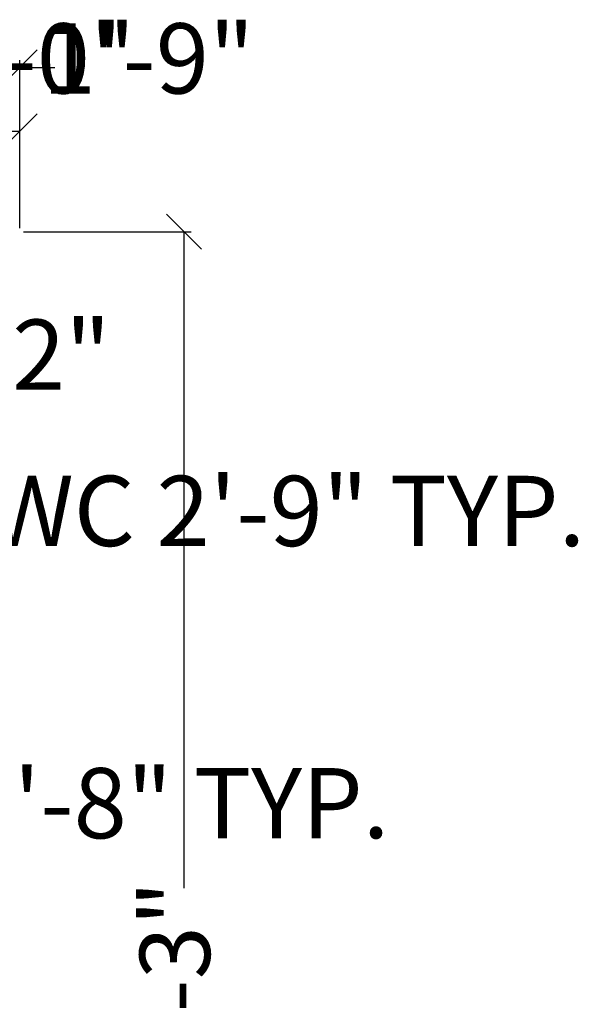
# Model space of a CAD drawing. Units: inches. Extents: x 2371 to 3019, y 129 to 700.
# Tile 14 of 14: x 2923 to 3019, y 499 to 667. Entities that reach past the tile are written whole.
import ezdxf

# ---------------------------------------------------------------- set-up
doc = ezdxf.new("R2010")
doc.units = ezdxf.units.IN
doc.layers.add('A-ANNO-DIMS', color=2, linetype='Continuous', lineweight=18)
doc.styles.get("Standard").update_dxf_attribs({"font": 'arial.ttf'})
doc.dimstyles.new('ISO-25', dxfattribs={"dimtxt": 12, "dimasz": 6, "dimexe": 1.25, "dimexo": 0.625, "dimtad": 0, "dimdec": 1, "dimlunit": 3, "dimtxsty": 'Standard', "dimblk": 'OBLIQUE', "dimblk1": 'ORIGIN2', "dimblk2": 'OBLIQUE', "dimcen": 2.5, "dimadec": 0, "dimazin": 0, "dimtfac": 1, "dimtdec": 1, "dimtmove": 0, "dimatfit": 3, "dimldrblk": 'OBLIQUE', "dimfxl": 1, "dimarcsym": 0})

# ---------------------------------------------------------------- blocks, each defined once
blk = doc.blocks.new('_Oblique')
at = {"color": 0, "linetype": 'ByBlock', "lineweight": -2}
blk.add_line((-0.5, -0.5), (0.5, 0.5), dxfattribs=at)
blk = doc.blocks.new('*D14')
at = {"layer": 'A-ANNO-DIMS', "color": 0, "lineweight": -2, "transparency": 16777216}
for p, q in [((2407.11, 631.6), (2407.11, 649.37)), ((2923.11, 631.6), (2923.11, 649.37)), ((2407.11, 648.12), (2643.63, 648.12)), ((2923.11, 648.12), (2686.58, 648.12))]:
    blk.add_line(p, q, dxfattribs=at)
at = {"layer": 'Defpoints', "color": 0, "lineweight": 25, "transparency": 16777216}
for p in [(2923.11, 648.12), (2407.11, 630.98), (2923.11, 630.98)]:
    blk.add_point(p, dxfattribs=at)
at = {"layer": 'A-ANNO-DIMS', "color": 0, "lineweight": -2, "transparency": 16777216, "xscale": 6, "yscale": 6, "zscale": 6, "rotation": 180}
blk.add_blockref('_Oblique', (2407.11, 648.12), dxfattribs=at)
at = {"layer": 'A-ANNO-DIMS', "color": 0, "lineweight": -2, "transparency": 16777216, "xscale": 6, "yscale": 6, "zscale": 6}
blk.add_blockref('_Oblique', (2923.11, 648.12), dxfattribs=at)
at = {"layer": 'A-ANNO-DIMS', "color": 0, "transparency": 16777216, "insert": (2665.11, 648.12), "char_height": 12, "width": 20.8486, "attachment_point": 5}
blk.add_mtext('43\'-0"', dxfattribs=at)
blk = doc.blocks.new('_Origin2')
at = {"color": 0, "linetype": 'ByBlock', "lineweight": -2}
blk.add_line((-0.5, 0), (-1, 0), dxfattribs=at)
for radius in [0.5, 0.25]:
    blk.add_circle((0, 0), radius, dxfattribs=at)
blk = doc.blocks.new('*D26')
at = {"layer": 'A-ANNO-DIMS', "color": 0, "lineweight": -2, "transparency": 16777216}
for p, q in [((2886.23, 560.02), (2881.92, 560.02)), ((2883.17, 560.02), (2883.17, 535.47)), ((2886.23, 535.47), (2881.92, 535.47)), ((2883.17, 535.47), (2883.17, 529.47))]:
    blk.add_line(p, q, dxfattribs=at)
at = {"layer": 'Defpoints', "color": 0, "lineweight": 25, "transparency": 16777216}
for p in [(2886.85, 560.02), (2883.17, 535.47), (2886.85, 535.47)]:
    blk.add_point(p, dxfattribs=at)
at = {"layer": 'A-ANNO-DIMS', "color": 0, "lineweight": -2, "transparency": 16777216, "xscale": 6, "yscale": 6, "zscale": 6}
for p, rotation in [((2883.17, 560.02), 90), ((2883.17, 535.47), 270)]:
    blk.add_blockref('_Oblique', p, dxfattribs=dict(at, rotation=rotation))
at = {"layer": 'A-ANNO-DIMS', "color": 0, "transparency": 16777216, "insert": (2883.17, 423.09), "char_height": 12, "attachment_point": 5, "rotation": 90}
blk.add_mtext('WASH BASIN 2\'-0 1/2" TYP.', dxfattribs=at)
blk = doc.blocks.new('*D27')
at = {"layer": 'A-ANNO-DIMS', "color": 0, "lineweight": -2, "transparency": 16777216}
for p, q in [((2886.85, 534.85), (2886.85, 530.54)), ((2906.99, 534.85), (2906.99, 530.54)), ((2886.85, 531.79), (2906.99, 531.79)), ((2906.99, 531.79), (2912.99, 531.79))]:
    blk.add_line(p, q, dxfattribs=at)
at = {"layer": 'Defpoints', "color": 0, "lineweight": 25, "transparency": 16777216}
for p in [(2886.85, 535.47), (2906.99, 535.47), (2906.99, 531.79)]:
    blk.add_point(p, dxfattribs=at)
at = {"layer": 'A-ANNO-DIMS', "color": 0, "lineweight": -2, "transparency": 16777216, "xscale": 6, "yscale": 6, "zscale": 6, "rotation": 180}
blk.add_blockref('_Oblique', (2886.85, 531.79), dxfattribs=at)
at = {"layer": 'A-ANNO-DIMS', "color": 0, "lineweight": -2, "transparency": 16777216, "xscale": 6, "yscale": 6, "zscale": 6}
blk.add_blockref('_Oblique', (2906.99, 531.79), dxfattribs=at)
at = {"layer": 'A-ANNO-DIMS', "color": 0, "transparency": 16777216, "insert": (2949.62, 531.79), "char_height": 12, "attachment_point": 5}
blk.add_mtext('1\'-8" TYP.', dxfattribs=at)
blk = doc.blocks.new('*D28')
at = {"layer": 'A-ANNO-DIMS', "color": 0, "lineweight": -2, "transparency": 16777216}
for p, q in [((2876.06, 586.05), (2876.06, 580.47)), ((2909.11, 586.05), (2909.11, 580.47)), ((2876.06, 581.72), (2909.11, 581.72)), ((2909.11, 581.72), (2915.11, 581.72))]:
    blk.add_line(p, q, dxfattribs=at)
at = {"layer": 'Defpoints', "color": 0, "lineweight": 25, "transparency": 16777216}
for p in [(2876.06, 586.68), (2909.11, 586.68), (2909.11, 581.72)]:
    blk.add_point(p, dxfattribs=at)
at = {"layer": 'A-ANNO-DIMS', "color": 0, "lineweight": -2, "transparency": 16777216, "xscale": 6, "yscale": 6, "zscale": 6, "rotation": 180}
blk.add_blockref('_Oblique', (2876.06, 581.72), dxfattribs=at)
at = {"layer": 'A-ANNO-DIMS', "color": 0, "lineweight": -2, "transparency": 16777216, "xscale": 6, "yscale": 6, "zscale": 6}
blk.add_blockref('_Oblique', (2909.11, 581.72), dxfattribs=at)
at = {"layer": 'A-ANNO-DIMS', "color": 0, "transparency": 16777216, "insert": (2968.84, 581.72), "char_height": 12, "attachment_point": 5}
blk.add_mtext('WC 2\'-9" TYP.', dxfattribs=at)
blk = doc.blocks.new('*D48')
at = {"layer": 'A-ANNO-DIMS', "color": 0, "lineweight": -2, "transparency": 16777216}
for p, q in [((2878.11, 631.6), (2878.11, 660.28)), ((2902.11, 631.6), (2902.11, 660.28)), ((2878.11, 659.03), (2902.11, 659.03)), ((2902.11, 659.03), (2908.11, 659.03))]:
    blk.add_line(p, q, dxfattribs=at)
at = {"layer": 'Defpoints', "color": 0, "lineweight": 25, "transparency": 16777216}
for p in [(2902.11, 659.03), (2878.11, 630.98), (2902.11, 630.98)]:
    blk.add_point(p, dxfattribs=at)
at = {"layer": 'A-ANNO-DIMS', "color": 0, "lineweight": -2, "transparency": 16777216, "xscale": 6, "yscale": 6, "zscale": 6, "rotation": 180}
blk.add_blockref('_Oblique', (2878.11, 659.03), dxfattribs=at)
at = {"layer": 'A-ANNO-DIMS', "color": 0, "lineweight": -2, "transparency": 16777216, "xscale": 6, "yscale": 6, "zscale": 6}
blk.add_blockref('_Oblique', (2902.11, 659.03), dxfattribs=at)
at = {"layer": 'A-ANNO-DIMS', "color": 0, "transparency": 16777216, "insert": (2924.78, 659.03), "char_height": 12, "attachment_point": 5}
blk.add_mtext('2\'-0"', dxfattribs=at)
blk = doc.blocks.new('*D49')
at = {"layer": 'A-ANNO-DIMS', "color": 0, "lineweight": -2, "transparency": 16777216}
for p, q in [((2902.11, 631.6), (2902.11, 660.28)), ((2923.11, 631.6), (2923.11, 660.28)), ((2902.11, 659.03), (2923.11, 659.03)), ((2923.11, 659.03), (2929.11, 659.03))]:
    blk.add_line(p, q, dxfattribs=at)
at = {"layer": 'Defpoints', "color": 0, "lineweight": 25, "transparency": 16777216}
for p in [(2923.11, 659.03), (2902.11, 630.98), (2923.11, 630.98)]:
    blk.add_point(p, dxfattribs=at)
at = {"layer": 'A-ANNO-DIMS', "color": 0, "lineweight": -2, "transparency": 16777216, "xscale": 6, "yscale": 6, "zscale": 6, "rotation": 180}
blk.add_blockref('_Oblique', (2902.11, 659.03), dxfattribs=at)
at = {"layer": 'A-ANNO-DIMS', "color": 0, "lineweight": -2, "transparency": 16777216, "xscale": 6, "yscale": 6, "zscale": 6}
blk.add_blockref('_Oblique', (2923.11, 659.03), dxfattribs=at)
at = {"layer": 'A-ANNO-DIMS', "color": 0, "transparency": 16777216, "insert": (2945.11, 659.03), "char_height": 12, "attachment_point": 5}
blk.add_mtext('1\'-9"', dxfattribs=at)
blk = doc.blocks.new('*D63')
at = {"layer": 'A-ANNO-DIMS', "color": 0, "lineweight": -2, "transparency": 16777216}
for p, q in [((2923.73, 630.98), (2952.41, 630.98)), ((2951.16, 630.98), (2951.16, 518.81)), ((2951.16, 363.98), (2951.16, 476.14)), ((2923.73, 363.98), (2952.41, 363.98))]:
    blk.add_line(p, q, dxfattribs=at)
at = {"layer": 'Defpoints', "color": 0, "lineweight": 25, "transparency": 16777216}
for p in [(2923.11, 630.98), (2951.16, 630.98), (2923.11, 363.98)]:
    blk.add_point(p, dxfattribs=at)
at = {"layer": 'A-ANNO-DIMS', "color": 0, "lineweight": -2, "transparency": 16777216, "xscale": 6, "yscale": 6, "zscale": 6}
for p, rotation in [((2951.16, 630.98), 90), ((2951.16, 363.98), 270)]:
    blk.add_blockref('_Oblique', p, dxfattribs=dict(at, rotation=rotation))
at = {"layer": 'A-ANNO-DIMS', "color": 0, "transparency": 16777216, "insert": (2951.16, 497.48), "char_height": 12, "attachment_point": 5, "rotation": 90}
blk.add_mtext('22\'-3"', dxfattribs=at)
blk = doc.blocks.new('*D77')
at = {"layer": 'A-ANNO-DIMS', "color": 0, "lineweight": -2, "transparency": 16777216}
for p, q in [((2838.11, 580.98), (2838.11, 609.66)), ((2869.78, 580.98), (2869.78, 609.66)), ((2838.11, 608.41), (2869.78, 608.41)), ((2869.78, 608.41), (2875.78, 608.41))]:
    blk.add_line(p, q, dxfattribs=at)
at = {"layer": 'Defpoints', "color": 0, "lineweight": 25, "transparency": 16777216}
for p in [(2869.78, 608.41), (2838.11, 580.36), (2869.78, 580.36)]:
    blk.add_point(p, dxfattribs=at)
at = {"layer": 'A-ANNO-DIMS', "color": 0, "lineweight": -2, "transparency": 16777216, "xscale": 6, "yscale": 6, "zscale": 6, "rotation": 180}
blk.add_blockref('_Oblique', (2838.11, 608.41), dxfattribs=at)
at = {"layer": 'A-ANNO-DIMS', "color": 0, "lineweight": -2, "transparency": 16777216, "xscale": 6, "yscale": 6, "zscale": 6}
blk.add_blockref('_Oblique', (2869.78, 608.41), dxfattribs=at)
at = {"layer": 'A-ANNO-DIMS', "color": 0, "transparency": 16777216, "insert": (2906.44, 608.41), "char_height": 12, "attachment_point": 5}
blk.add_mtext('2\'-7 1/2"', dxfattribs=at)

msp = doc.modelspace()

# ---------------------------------------------------------------- dimensions: what is measured, and where the dimension line sits
at = {"layer": 'A-ANNO-DIMS'}
for base, p1, p2, picture, middle in [((2902.11, 659.03), (2878.11, 630.98), (2902.11, 630.98), '*D48', (2924.78, 659.03)), ((2923.11, 659.03), (2902.11, 630.98), (2923.11, 630.98), '*D49', (2945.11, 659.03))]:
    dim = msp.add_linear_dim(base=base, p1=p1, p2=p2, dimstyle='ISO-25', override={"dimdec": 1, "dimlfac": 1, "dimrnd": 0, "dimzin": 1, "dimdsep": 46, "dimlunit": 4, "dimfrac": 2}, dxfattribs=at)
    dim.commit()
    dim.dimension.update_dxf_attribs({"geometry": picture, "text_midpoint": middle})
for base, p1, p2, text, override, picture, middle in [((2923.11, 648.12), (2407.11, 630.98), (2923.11, 630.98), '43\'-0"', {"dimclrd": 0, "dimclre": 0, "dimclrt": 0}, '*D14', (2665.11, 648.12)), ((2909.1051, 581.7183), (2876.0589, 586.6753), (2909.1051, 586.6753), 'WC <> TYP.', {"dimdec": 1, "dimrnd": 0, "dimzin": 1, "dimlunit": 4, "dimfrac": 2}, '*D28', (2968.842, 581.7183)), ((2906.99, 531.79), (2886.85, 535.47), (2906.99, 535.47), '<> TYP.', {"dimdec": 1, "dimrnd": 0, "dimzin": 1, "dimlunit": 4, "dimfrac": 2}, '*D27', (2949.62, 531.79))]:
    dim = msp.add_linear_dim(base=base, p1=p1, p2=p2, text=text, dimstyle='ISO-25', override=override, dxfattribs=at)
    dim.commit()
    dim.dimension.update_dxf_attribs({"geometry": picture, "text_midpoint": middle})
for base, p1, p2, angle, picture, middle in [((2951.16, 630.98), (2923.11, 363.98), (2923.11, 630.98), 90, '*D63', (2951.16, 497.48)), ((2869.78, 608.41), (2838.11, 580.36), (2869.78, 580.36), 0, '*D77', (2906.44, 608.41))]:
    dim = msp.add_linear_dim(base=base, p1=p1, p2=p2, angle=angle, dimstyle='ISO-25', override={"dimdec": 1, "dimlfac": 1, "dimrnd": 0, "dimzin": 1, "dimdsep": 46, "dimlunit": 4, "dimfrac": 2}, dxfattribs=at)
    dim.commit()
    dim.dimension.update_dxf_attribs({"geometry": picture, "text_midpoint": middle})
dim = msp.add_linear_dim(base=(2883.1676, 535.4732), p1=(2886.8502, 560.0241), p2=(2886.8502, 535.4732), angle=270, text='WASH BASIN <> TYP.', dimstyle='ISO-25', override={"dimdec": 1, "dimrnd": 0, "dimzin": 1, "dimlunit": 4, "dimfrac": 2}, dxfattribs=at)
dim.commit()
dim.dimension.update_dxf_attribs({"geometry": '*D26', "text_midpoint": (2883.1676, 423.0911)})

doc.saveas('drawing.dxf')
